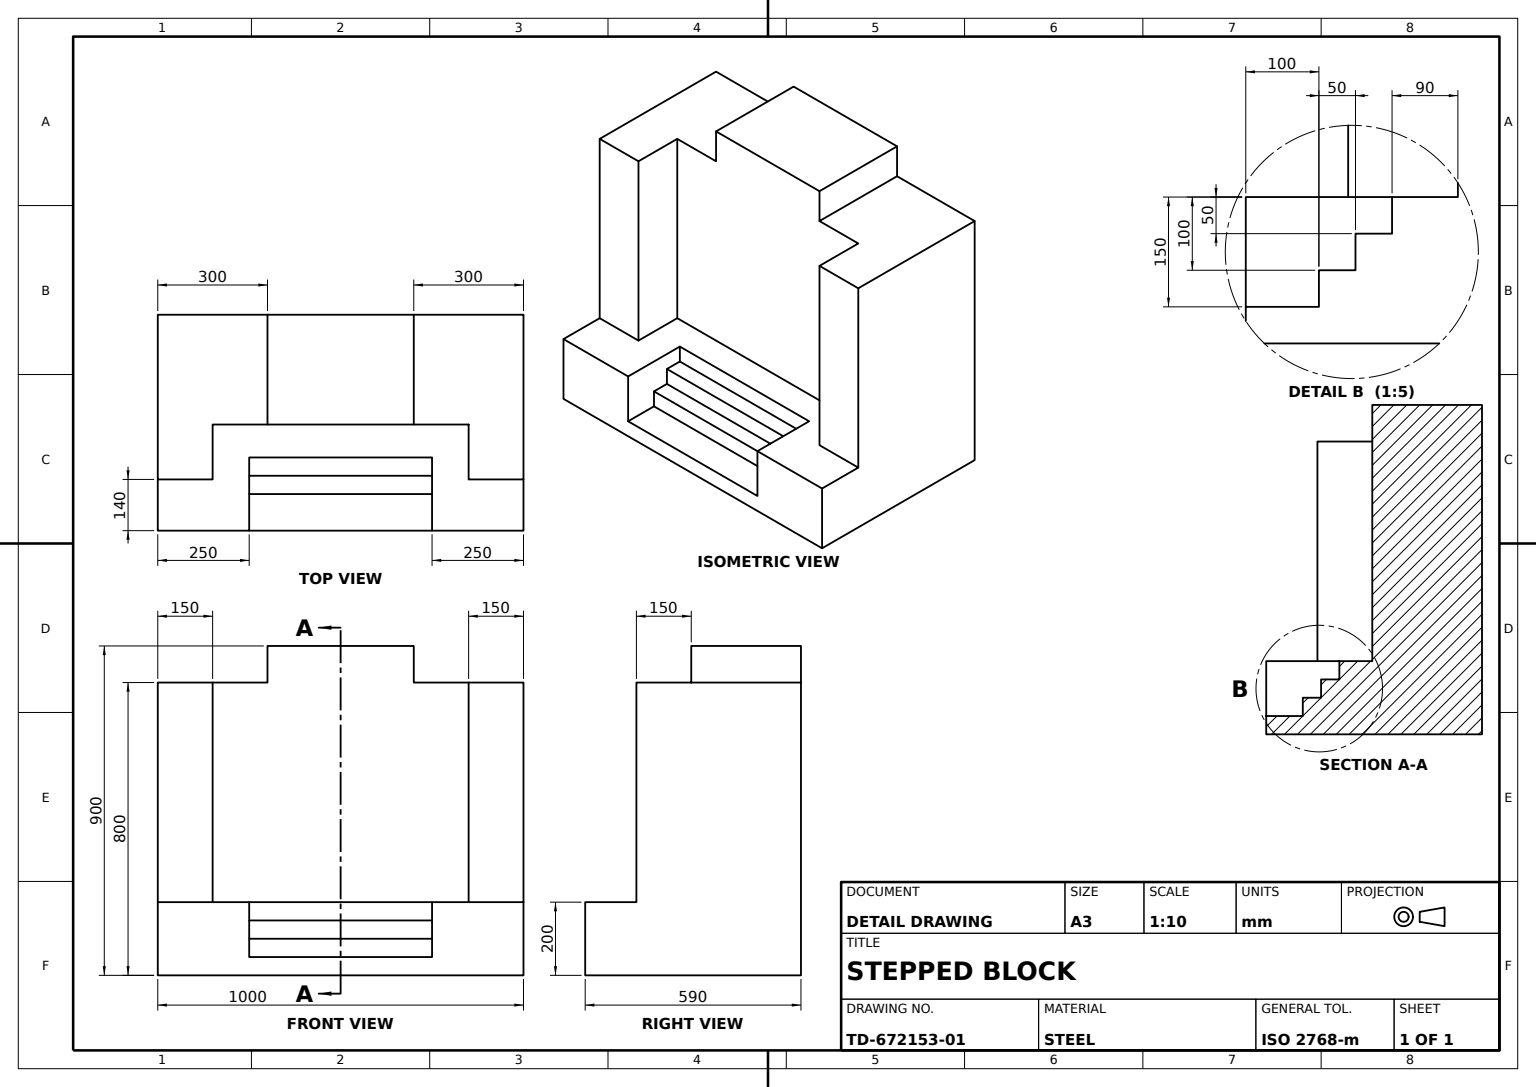
SolidWorks part; units mm, degrees
material "Plain Carbon Steel"
ref_plane "Front Plane" through (0, 0, 0) normal (0, 0, 1) x (1, 0, 0)
ref_plane "Top Plane" through (0, 0, 0) normal (0, 1, 0) x (1, 0, 0)
ref_plane "Right Plane" through (0, 0, 0) normal (1, 0, 0) x (0, 0, -1)
sketch "Base Profile Sketch" plane through (0, 0, 0) normal (0, 0, 1) x (1, 0, 0)
  line L0 (0, 0) -> (540, 0)
  line L1 (540, 0) -> (540, 800)
  line L2 (540, 800) -> (240, 800)
  line L3 (240, 800) -> (240, 200)
  line L4 (240, 200) -> (0, 200)
  line L5 (0, 200) -> (0, 0)
  dimension "D1" = 240
  dimension "D2" = 540
  dimension "D3" = 200
  dimension "D4" = 800
extrude "Base Block" add sketch "Base Profile Sketch" along normal blind 1000
sketch "Side Boss A Sketch" plane through (0, 0, 0) normal (0, 0, -1) x (-1, 0, 0)
  line L0 (-240, 800) -> (-90, 800)
  line L1 (-90, 800) -> (-90, 200)
  line L2 (-240, 200) -> (0, 200) construction
  line L3 (-90, 200) -> (-240, 200)
  line L4 (-240, 800) -> (-240, 200) construction
  line L5 (-240, 200) -> (-240, 800)
  line L6 (0, 200) -> (0, 0) construction
  dimension "D1" = 90
extrude "Side Boss A" add sketch "Side Boss A Sketch" against normal blind 150
sketch "Side Boss B Sketch" plane through (0, 0, 1000) normal (0, 0, 1) x (1, 0, 0)
  line L0 (240, 800) -> (240, 200)
  line L1 (240, 200) -> (90, 200)
  line L2 (90, 200) -> (90, 800)
  line L3 (90, 800) -> (240, 800)
extrude "Side Boss B" add sketch "Side Boss B Sketch" against normal blind 150
sketch "Corner Boss Sketch" plane through (0, 800, 0) normal (0, 1, 0) x (1, 0, 0)
  line L0 (540, -1000) -> (540, 0) construction
  line L1 (540, -1000) -> (90, -1000) construction
  line L3 (540, -500) -> (540, -300)
  line L4 (540, -300) -> (240, -300)
  line L5 (240, -850) -> (240, -150) construction
  line L6 (240, -300) -> (240, -700)
  line L7 (240, -700) -> (540, -700)
  line L8 (540, -700) -> (540, -500)
  line L9 (540, 0) -> (90, 0) construction
  dimension "D1" = 300
  dimension "D2" = 300
extrude "Corner Boss" add sketch "Corner Boss Sketch" along normal blind 100
sketch "Top Step Cut Sketch" plane through (0, 0, 0) normal (-1, 0, 0) x (0, 0, 1)
  line L0 (0, 200) -> (0, 0) construction
  line L1 (1000, 0) -> (0, 0) construction
  line L2 (850, 200) -> (150, 200) construction
  line L3 (500, 200) -> (250, 200)
  line L4 (1000, 200) -> (0, 200) construction
  line L5 (250, 200) -> (250, 150)
  line L6 (250, 150) -> (750, 150)
  line L7 (750, 150) -> (750, 200)
  line L8 (750, 200) -> (500, 200)
  dimension "D1" = 250
  dimension "D2" = 150
extrude "Top Step Cut" cut sketch "Top Step Cut Sketch" against normal blind 150
sketch "Top Groove Sketch" plane through (0, 0, 0) normal (-1, 0, 0) x (0, 0, 1)
  line L0 (250, 150) -> (250, 100)
  line L1 (250, 100) -> (750, 100)
  line L2 (750, 100) -> (750, 150)
  line L4 (250, 150) -> (750, 150) construction
  dimension "D1" = 50
extrude "Top Groove Cut" cut sketch "Top Groove Sketch" against normal blind 100 and the other way through all
sketch "Groove Notch Sketch" plane through (0, 0, 0) normal (-1, 0, 0) x (0, 0, 1)
  line L0 (250, 100) -> (250, 50)
  line L1 (250, 50) -> (750, 50)
  line L2 (750, 50) -> (750, 100)
  line L3 (750, 100) -> (250, 100)
  line L5 (750, 100) -> (250, 100) construction
  dimension "D1" = 50
extrude "Groove Notch Cut" cut sketch "Groove Notch Sketch" against normal blind 50
sketch "Groove Infill Sketch" plane through (0, 0, 0) normal (-1, 0, 0) x (0, 0, 1)
  line L0 (0, 200) -> (0, 0)
  line L1 (0, 0) -> (1000, 0)
  line L2 (1000, 0) -> (1000, 200)
  line L3 (1000, 200) -> (750, 200)
  line L4 (750, 50) -> (750, 200) construction
  line L5 (1000, 200) -> (750, 200) construction
  line L6 (750, 200) -> (750, 50)
  line L7 (250, 50) -> (750, 50) construction
  line L8 (250, 50) -> (750, 50) construction
  line L9 (750, 50) -> (250, 50)
  line L10 (250, 50) -> (250, 200)
  line L11 (850, 200) -> (150, 200) construction
  line L12 (250, 200) -> (0, 200)
extrude "Groove Infill Boss" add sketch "Groove Infill Sketch" along normal blind 50
